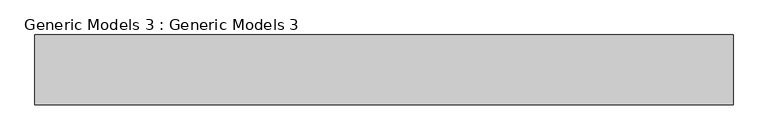
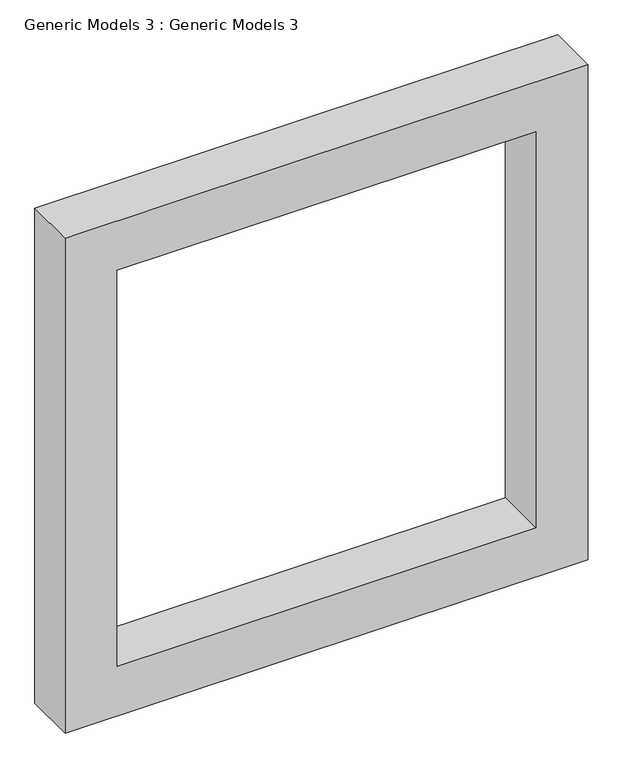
"""IFC4 building model written with IfcOpenShell, lengths in millimetres: proxy geometry, Generic Models 3 : Generic Models 3."""

from ifc_helpers import new_model, si_unit, frame, origin, place, context, project, spatial, polyline, outline, extrude, source, transform, mapped, element, save


def generic_models_3_generic_models_3_0ad4c425(model_context):
    return source(origin(), model_context, "Body", "SweptSolid", [
        extrude(outline(polyline([(5943.6, -6239.0023867), (5943.6, -7763.0023867), (4419.6, -7763.0023867), (4419.6, -6239.0023867), (5943.6, -6239.0023867)]), holes=[polyline([(5791.2, -6391.4023867), (4572.0, -6391.4023867), (4572.0, -7610.6023867), (5791.2, -7610.6023867), (5791.2, -6391.4023867)])]), frame((0.0, -1994.7499863, 0.0), z_axis=(0.0, 1.0, 0.0), x_axis=(0.0, 0.0, 1.0)), (0.0, 0.0, 1.0), 152.4),
    ])


if __name__ == "__main__":
    model = new_model("IFC4")
    model_context = context("Model", 3, world=origin())
    ifc_project = project(units=[si_unit("LENGTHUNIT", "METRE", prefix="MILLI")], contexts=[model_context])
    site = spatial("IfcSite", under=ifc_project)
    building = spatial("IfcBuilding", under=site)
    placement = place(None, origin())
    generic_models_3_generic_models_3_shape = generic_models_3_generic_models_3_0ad4c425(model_context)
    element("IfcBuildingElementProxy", 1, Name="Generic Models 3 : Generic Models 3", ObjectType="Generic Models 3 : Generic Models 3", at=placement, inside=building, context=model_context, shape_type="MappedRepresentation", body=[
        mapped(generic_models_3_generic_models_3_shape, transform((0.0, 0.0, 0.0), x_axis=(1.0, 0.0, 0.0), y_axis=(0.0, 1.0, 0.0), z_axis=(0.0, 0.0, 1.0))),
    ])
    save(model, "model.ifc")

# Revit data of these elements
# Element 1 (IfcBuildingElementProxy, "Generic Models 3 : Generic Models 3")
#   Materials on its faces: "accent wall"
# Materials
#   "accent wall": class "Generic", colour RGB 120 120 120, transparency 0, Cost = 0
